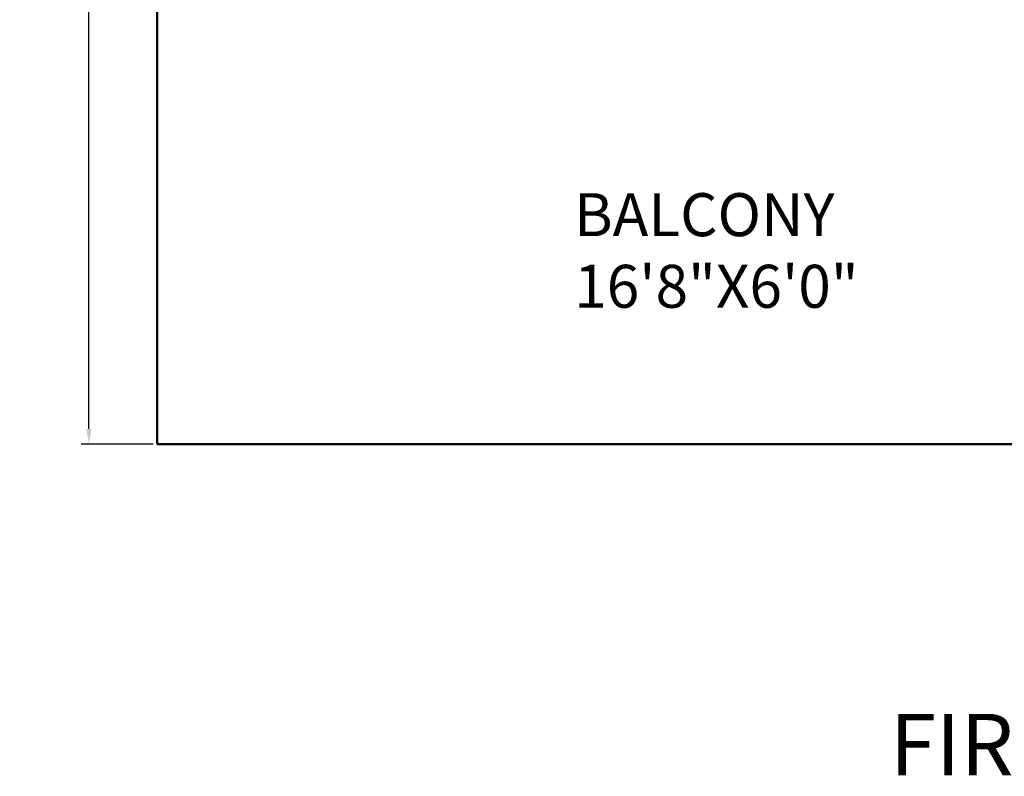
# Model space of a CAD drawing. Units: inches. Extents: x 3064 to 19385, y 846 to 15425.
# Tile 10 of 108: x 3625 to 3785, y 850 to 974. Entities that reach past the tile are written whole.
import ezdxf

# ---------------------------------------------------------------- set-up
doc = ezdxf.new("R2010")
doc.units = ezdxf.units.IN
for name, color, linetype, lineweight in [('A-ANNO-DIMS', 2, 'Continuous', 18), ('A-ANNO-TEXT', 7, 'Continuous', 25), ('A-AREA-IDEN', 3, 'Continuous', 18), ('A-WALL', 7, 'Continuous', 50)]:
    doc.layers.add(name, color=color, linetype=linetype, lineweight=lineweight)
doc.styles.get("Standard").update_dxf_attribs({"font": 'arial.ttf'})
doc.dimstyles.new('ISO-25', dxfattribs={"dimtxt": 9, "dimasz": 2.5, "dimexe": 1.25, "dimexo": 0.625, "dimtad": 1, "dimdec": 1, "dimlunit": 3, "dimtxsty": 'Standard', "dimcen": 2.5, "dimadec": 0, "dimazin": 0, "dimtfac": 1, "dimtdec": 1, "dimtmove": 0, "dimatfit": 3, "dimfxl": 1, "dimarcsym": 0})

# ---------------------------------------------------------------- blocks, each defined once
blk = doc.blocks.new('*D40')
at = {"layer": 'A-ANNO-DIMS', "color": 0, "lineweight": -2, "transparency": 16777216}
for p, q in [((3646.73, 1396.34), (3634.99, 1396.34)), ((3636.24, 906.84), (3636.24, 1393.84)), ((3646.73, 904.34), (3634.99, 904.34))]:
    blk.add_line(p, q, dxfattribs=at)
at = {"layer": 'A-ANNO-DIMS', "color": 0, "transparency": 16777216}
for points in [[(3635.82, 1393.84), (3636.66, 1393.84), (3636.24, 1396.34)], [(3635.82, 906.84), (3636.66, 906.84), (3636.24, 904.34)]]:
    blk.add_solid(points, dxfattribs=at)
at = {"layer": 'Defpoints', "color": 0, "transparency": 16777216}
for p in [(3636.24, 1396.34), (3647.36, 1396.34), (3647.36, 904.34)]:
    blk.add_point(p, dxfattribs=at)
at = {"layer": 'A-ANNO-DIMS', "color": 0, "transparency": 16777216, "insert": (3631.1, 1150.34), "char_height": 9, "attachment_point": 5, "rotation": 90}
blk.add_mtext("41'", dxfattribs=at)

msp = doc.modelspace()

# ---------------------------------------------------------------- linework, layer by layer
at = {"layer": 'A-WALL'}
for p, q in [((3647.36, 976.34), (3647.36, 904.34)), ((3647.36, 904.34), (3989.36, 904.34))]:
    msp.add_line(p, q, dxfattribs=at)

# ---------------------------------------------------------------- texts
at = {"layer": 'A-ANNO-TEXT', "insert": (3766.7, 860.41), "char_height": 10, "attachment_point": 1}
msp.add_mtext_dynamic_manual_height_columns('FIRST FLOOR PLAN', width=200.9739, gutter_width=12.5, heights=[0], dxfattribs=at)
at = {"layer": 'A-AREA-IDEN', "insert": (3715.29, 945.24), "char_height": 7, "attachment_point": 1}
msp.add_mtext_dynamic_manual_height_columns('BALCONY\\P16\'8"X6\'0"', width=67.5924, gutter_width=12.5, heights=[0], dxfattribs=at)

# ---------------------------------------------------------------- dimensions: what is measured, and where the dimension line sits
at = {"layer": 'A-ANNO-DIMS'}
dim = msp.add_linear_dim(base=(3636.24, 1396.34), p1=(3647.36, 904.34), p2=(3647.36, 1396.34), angle=90, dimstyle='ISO-25', override={"dimclrd": 0, "dimclre": 0, "dimclrt": 0}, dxfattribs=at)
dim.commit()
dim.dimension.update_dxf_attribs({"geometry": '*D40', "text_midpoint": (3631.1, 1150.34)})

doc.saveas('drawing.dxf')
